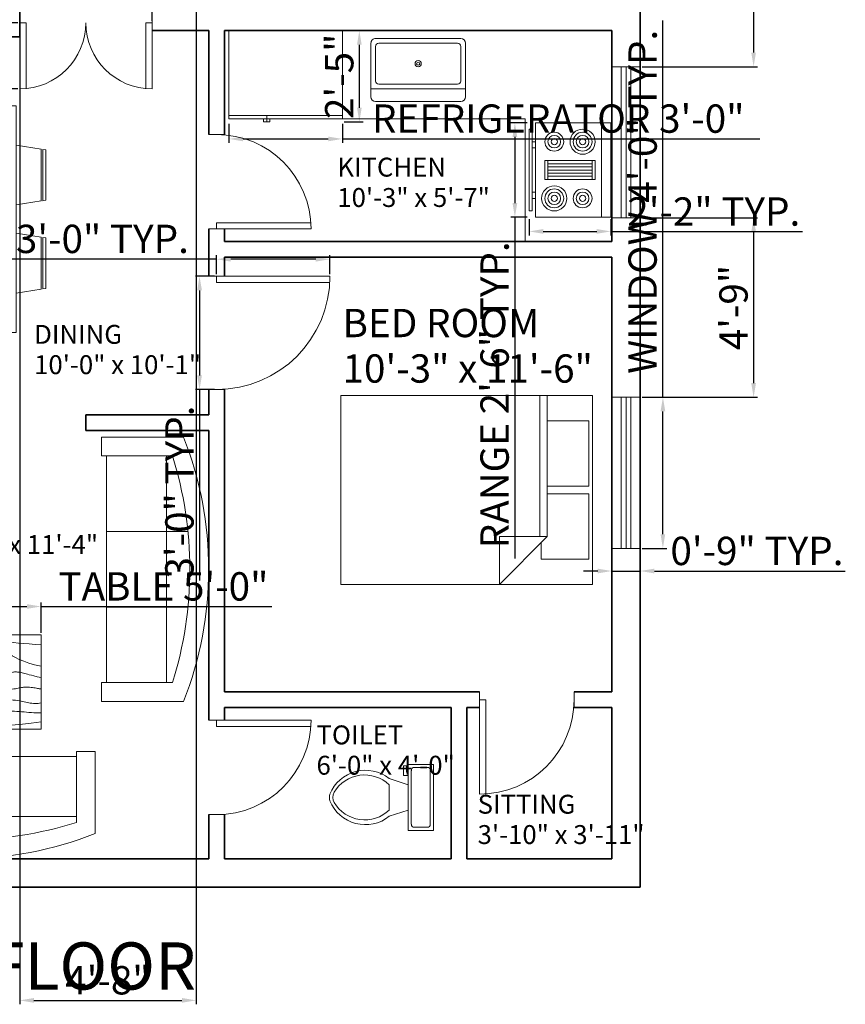
# Model space of a CAD drawing. Units: inches. Extents: x 3087 to 8148, y 1377 to 3709.
# Tile 4 of 6: x 3443 to 3705, y 1377 to 1689. Entities that reach past the tile are written whole.
import ezdxf

# ---------------------------------------------------------------- set-up
doc = ezdxf.new("R2010")
doc.units = ezdxf.units.IN
for name, color, linetype, lineweight, true_color in [('A-ANNO-DIMS', 244, 'Continuous', 18, 0x991b1e), ('A-ANNO-TEXT', 244, 'Continuous', 25, 0x991b1e), ('A-AREA-IDEN', 244, 'Continuous', 18, 0x991b1e), ('A-DOOR', 146, 'Continuous', 18, 0x105689), ('A-GLAZ', 146, 'Continuous', 18, 0x105689), ('A-WALL', 241, 'Continuous', 35, 0xf7abae)]:
    doc.layers.add(name, color=color, linetype=linetype, lineweight=lineweight, true_color=true_color)
for name, color, linetype, lineweight in [('A-EQPM', 8, 'Continuous', 18), ('A-FLOR-CASE', 9, 'Continuous', 18), ('A-FLOR-FIXT', 9, 'Continuous', 18), ('A-FURN', 8, 'Continuous', 18)]:
    doc.layers.add(name, color=color, linetype=linetype, lineweight=lineweight)
doc.styles.get("Standard").update_dxf_attribs({"font": 'arial.ttf'})
doc.dimstyles.new('ISO-25', dxfattribs={"dimtxt": 9, "dimasz": 4.5, "dimexe": 1.25, "dimexo": 0.625, "dimtad": 1, "dimdec": 0, "dimlunit": 3, "dimtxsty": 'Standard', "dimcen": 2.5, "dimadec": 0, "dimazin": 0, "dimtfac": 1, "dimtdec": 0, "dimtmove": 0, "dimatfit": 3, "dimfxl": 1, "dimarcsym": 0})

# ---------------------------------------------------------------- blocks, each defined once
blk = doc.blocks.new('Bed - Queen')
for p, q in [((0, -80.00003), (0, 0)), ((0, 0), (59.99999, 0)), ((59.99999, 0), (59.99999, -80.00003)), ((7.99999, -1.2), (28.79998, -1.2)), ((7.99999, -14.4), (7.99999, -1.2)), ((28.79998, -1.2), (28.79998, -14.4)), ((31.19999, -1.2), (51.99999, -1.2)), ((31.19999, -14.4), (31.19999, -1.2)), ((51.99999, -1.2), (51.99999, -16.4)), ((0, -14.4), (44.8, -14.4)), ((59.99999, -29.6), (44.8, -14.4)), ((44.8, -14.4), (44.8, -29.6)), ((44.8, -16.8), (0, -16.8)), ((51.99999, -16.4), (46.79936, -16.4)), ((44.8, -29.6), (59.99999, -29.6)), ((59.99999, -80.00003), (0, -80.00003))]:
    blk.add_line(p, q)
blk = doc.blocks.new('Sofa - Roundback 7 ft.')
for p, q in [((-12.00002, -32.4421), (-12.00003, -6.5971)), ((11.99997, -32.4421), (11.99998, -6.5971)), ((-36.000027, -34), (-36.000027, -11.4696)), ((35.99998, -34), (35.99998, -11.4696)), ((-35.999844, -13.3819), (35.9998, -13.3819)), ((-36.000027, -32.4421), (35.99998, -32.4421))]:
    blk.add_line(p, q)
for points in [[(-36.000027, -34), (-42.000027, -34), (-42.000027, -8)], [(41.99998, -8), (41.99998, -34), (35.99998, -34)]]:
    blk.add_lwpolyline(points)
for centre, radius, start, end in [((0, -114.25), 114.25, 68.43141, 111.5686), ((-0.00001, -127.1968), 121.1968, 72.72033, 107.2797)]:
    blk.add_arc(centre, radius, start, end)
blk = doc.blocks.new('Table - Rectangular Woodgrain 60 x 30 in.')
for p, q in [((0, 0), (0, -30)), ((60, 0), (0, 0)), ((60, -30), (60, 0)), ((0, -30), (60, -30))]:
    blk.add_line(p, q)
for points in [[(0, -2.4), (4.8155, -2.418), (9.0302, -2.4688), (12.709, -2.5477), (15.9167, -2.65), (18.7181, -2.7711), (21.1781, -2.9063), (23.3616, -3.0508), (25.3333, -3.2), (27.1477, -3.3495), (28.8172, -3.4958), (30.3437, -3.636), (31.7291, -3.7667), (32.9756, -3.8849), (34.0849, -3.9875), (35.059, -4.0714), (35.9, -4.1334), (36.6114, -4.1711), (37.2041, -4.1854), (37.6906, -4.1779), (38.0833, -4.15), (38.3948, -4.1034), (38.6375, -4.0396), (38.8239, -3.9602), (38.9666, -3.8667), (39.0764, -3.7608), (39.1573, -3.6448), (39.2116, -3.521), (39.2416, -3.3917), (39.2498, -3.2593), (39.2385, -3.1261), (39.21, -2.9944), (39.1666, -2.8667), (39.111, -2.7447), (39.0468, -2.6281), (38.978, -2.5163), (38.9083, -2.4083), (38.8418, -2.3035), (38.7823, -2.201), (38.7337, -2.1001), (38.7, -2), (38.6844, -1.9003), (38.6875, -1.8021), (38.7094, -1.707), (38.75, -1.6167), (38.8094, -1.5326), (38.8875, -1.4563), (38.9844, -1.3893), (39.1, -1.3333), (39.2351, -1.2896), (39.3937, -1.2583), (39.5804, -1.2396), (39.8, -1.2333), (40.057, -1.2396), (40.3562, -1.2583), (40.7023, -1.2896), (41.1, -1.3333), (41.5547, -1.3895), (42.0755, -1.4573), (42.6721, -1.5361), (43.3542, -1.625), (44.1316, -1.7233), (45.014, -1.8302), (46.0114, -1.9449), (47.1333, -2.0667), (48.3862, -2.1947), (49.7625, -2.3281), (51.2513, -2.4663), (52.8416, -2.6083), (54.5226, -2.7535), (56.2833, -2.9011), (58.1127, -3.0501), (60, -3.2)], [(0, -9.2), (6.5759, -9.0858), (11.9385, -9.0365), (16.2527, -9.0418), (19.6833, -9.0917), (22.3952, -9.1759), (24.5531, -9.2844), (26.322, -9.4069), (27.8666, -9.5333), (29.3241, -9.6553), (30.7203, -9.7719), (32.0532, -9.8837), (33.3208, -9.9917), (34.5213, -10.0965), (35.6526, -10.199), (36.7128, -10.2999), (37.7, -10.4), (38.6129, -10.4996), (39.4531, -10.5969), (40.223, -10.6895), (40.925, -10.775), (41.5613, -10.8512), (42.1344, -10.9156), (42.6465, -10.966), (43.1, -11), (43.4976, -11.0158), (43.8437, -11.0136), (44.143, -10.9942), (44.4, -10.9583), (44.6195, -10.9069), (44.8062, -10.8406), (44.9648, -10.7603), (45.1, -10.6667), (45.2155, -10.5598), (45.3114, -10.4365), (45.3871, -10.2929), (45.4416, -10.125), (45.4743, -9.929), (45.4844, -9.7011), (45.4709, -9.4371), (45.4333, -9.1333), (45.3716, -8.7883), (45.2896, -8.4104), (45.1919, -8.0107), (45.0833, -7.6), (44.9685, -7.1893), (44.8521, -6.7896), (44.7388, -6.4117), (44.6333, -6.0667), (44.54, -5.7628), (44.4614, -5.4979), (44.4001, -5.2675), (44.3583, -5.0667), (44.3384, -4.8909), (44.3427, -4.7354), (44.3736, -4.5956), (44.4333, -4.4667), (44.5236, -4.3453), (44.6427, -4.2333), (44.7884, -4.1339), (44.9583, -4.05), (45.1501, -3.9849), (45.3614, -3.9417), (45.59, -3.9234), (45.8333, -3.9333), (46.0915, -3.9749), (46.3734, -4.0531), (46.6906, -4.1736), (47.0542, -4.3417), (47.4756, -4.5629), (47.9661, -4.8427), (48.5372, -5.1866), (49.2, -5.6), (49.9676, -6.0844), (50.8594, -6.625), (51.8965, -7.2031), (53.1, -7.8), (54.491, -8.3969), (56.0906, -8.975), (57.9199, -9.5156), (60, -10)], [(0, -12.8), (5.1847, -12.9322), (9.6213, -13.0323), (13.3963, -13.1059), (16.5958, -13.1583), (19.3063, -13.1952), (21.614, -13.2219), (23.6054, -13.2439), (25.3666, -13.2667), (26.9728, -13.2947), (28.4531, -13.3281), (29.8256, -13.3663), (31.1083, -13.4083), (32.3191, -13.4535), (33.476, -13.501), (34.597, -13.5501), (35.7, -13.6), (36.7984, -13.6497), (37.8875, -13.6979), (38.9578, -13.743), (40, -13.7833), (41.0047, -13.8174), (41.9625, -13.8438), (42.864, -13.8607), (43.7, -13.8667), (44.4631, -13.8604), (45.1552, -13.8417), (45.7801, -13.8104), (46.3416, -13.7667), (46.8439, -13.7104), (47.2906, -13.6417), (47.6858, -13.5604), (48.0333, -13.4667), (48.3375, -13.3608), (48.6042, -13.2448), (48.8396, -13.121), (49.05, -12.9917), (49.2417, -12.8593), (49.4208, -12.7261), (49.5937, -12.5944), (49.7667, -12.4667), (49.9452, -12.3451), (50.1323, -12.2313), (50.3303, -12.1268), (50.5416, -12.0333), (50.7686, -11.9524), (51.0135, -11.8854), (51.2788, -11.8341), (51.5666, -11.8), (51.8785, -11.7843), (52.2116, -11.7865), (52.562, -11.8059), (52.926, -11.8417), (53.2998, -11.8931), (53.6795, -11.9594), (54.0614, -12.0397), (54.4416, -12.1333), (54.8223, -12.2401), (55.2293, -12.3625), (55.6942, -12.5037), (56.2489, -12.6667), (56.9251, -12.8547), (57.7545, -13.0708), (58.7689, -13.3182), (60, -13.6)], [(0, -18), (5.124, -17.7273), (9.6609, -17.5057), (13.6705, -17.3303), (17.2125, -17.1958), (20.3467, -17.0973), (23.1328, -17.0297), (25.6307, -16.9878), (27.9, -16.9667), (29.9928, -16.9617), (31.9302, -16.9703), (33.7254, -16.9907), (35.3917, -17.0208), (36.9423, -17.0588), (38.3906, -17.1026), (39.7499, -17.1503), (41.0333, -17.2), (42.2519, -17.2496), (43.4073, -17.2969), (44.4986, -17.3395), (45.525, -17.375), (46.4858, -17.4012), (47.3802, -17.4156), (48.2074, -17.416), (48.9667, -17.4), (49.6583, -17.3662), (50.2872, -17.3167), (50.8595, -17.2547), (51.3812, -17.1833), (51.8584, -17.1057), (52.2971, -17.025), (52.7034, -16.9443), (53.0833, -16.8667), (53.443, -16.7951), (53.789, -16.7313), (54.128, -16.6768), (54.4666, -16.6334), (54.8115, -16.6024), (55.1693, -16.5854), (55.5465, -16.5841), (55.95, -16.6), (56.3828, -16.6337), (56.8346, -16.6823), (57.2915, -16.7418), (57.7396, -16.8084), (58.165, -16.878), (58.5539, -16.9469), (58.8924, -17.0111), (59.1666, -17.0667), (59.3679, -17.1107), (59.5078, -17.1438), (59.6032, -17.1675), (59.6708, -17.1833), (59.7275, -17.193), (59.7901, -17.1979), (59.8753, -17.1998), (60, -17.2)], [(0, -22.4), (8.0098, -22.2501), (14.4094, -22.1011), (19.4168, -21.9535), (23.25, -21.8083), (26.1269, -21.6663), (28.2656, -21.5281), (29.884, -21.3947), (31.2, -21.2667), (32.3967, -21.1448), (33.5172, -21.0292), (34.5697, -20.9198), (35.5625, -20.8167), (36.5037, -20.7198), (37.4015, -20.6292), (38.2642, -20.5448), (39.1, -20.4667), (39.9164, -20.3951), (40.7187, -20.3313), (41.5117, -20.2768), (42.3, -20.2333), (43.0883, -20.2024), (43.8812, -20.1854), (44.6836, -20.1841), (45.5, -20.2), (46.3328, -20.234), (47.1747, -20.2844), (48.0163, -20.3488), (48.8479, -20.425), (49.66, -20.5106), (50.4429, -20.6031), (51.1872, -20.7004), (51.8833, -20.8), (52.5246, -20.8999), (53.1166, -20.9995), (53.6681, -21.0983), (54.1875, -21.1958), (54.6834, -21.2919), (55.1646, -21.3859), (55.6394, -21.4777), (56.1167, -21.5667), (56.6028, -21.6515), (57.0961, -21.7266), (57.5929, -21.7852), (58.0896, -21.8208), (58.5823, -21.8268), (59.0674, -21.7964), (59.5412, -21.723), (60, -21.6)], [(0, -25.2), (8.6355, -25.0504), (15.7026, -24.9031), (21.4049, -24.7606), (25.9458, -24.625), (29.529, -24.4988), (32.3578, -24.3844), (34.6359, -24.284), (36.5667, -24.2), (38.3213, -24.1341), (39.9417, -24.0854), (41.437, -24.0523), (42.8167, -24.0333), (44.0901, -24.0268), (45.2667, -24.0313), (46.3557, -24.0451), (47.3667, -24.0667), (48.309, -24.0947), (49.1928, -24.1287), (50.0284, -24.168), (50.826, -24.2125), (51.5959, -24.2617), (52.3483, -24.3151), (53.0935, -24.3725), (53.8417, -24.4334), (54.6009, -24.497), (55.3699, -24.561), (56.1454, -24.6226), (56.9239, -24.6792), (57.7021, -24.7279), (58.4764, -24.7662), (59.2435, -24.7911), (60, -24.8)], [(0, -28.8), (5.6867, -28.6681), (10.45, -28.5698), (14.407, -28.5012), (17.675, -28.4584), (20.3711, -28.4374), (22.6125, -28.4344), (24.5164, -28.4455), (26.2, -28.4667), (27.762, -28.4947), (29.2276, -28.5281), (30.6033, -28.5663), (31.8958, -28.6084), (33.1118, -28.6535), (34.2578, -28.7011), (35.3405, -28.7501), (36.3666, -28.8), (37.3443, -28.8497), (38.288, -28.8974), (39.2137, -28.9412), (40.1375, -28.9792), (41.0753, -29.0093), (42.0432, -29.0297), (43.0572, -29.0384), (44.1333, -29.0333), (45.2936, -29.0114), (46.5843, -28.9641), (48.0579, -28.8816), (49.7666, -28.7542), (51.7629, -28.5721), (54.0989, -28.3255), (56.8272, -28.0048), (60, -27.6)]]:
    blk.add_lwpolyline(points)
blk = doc.blocks.new('Toilet - top')
for p, q in [((9.5, -6), (9.5, -2)), ((-10, -8.5), (-8, -8.5)), ((-10, -9.5), (-10, -8.5)), ((-8, -8.5), (-8, -8)), ((-7, -8), (-7, -9.5)), ((-4, -8), (-6, -14)), ((4, -8), (6, -14)), ((-7, -9.5), (-10, -9.5)), ((4, -14), (-4, -14))]:
    blk.add_line(p, q)
blk.add_lwpolyline([(10.5, -8), (10.5, 0), (-10.5, 0), (-10.5, -8)], close=True)
for points in [[(-9.5, -2), (-9.5, -6)], [(8.5, -1), (-8.5, -1)], [(-8.5, -7), (8.5, -7)]]:
    blk.add_lwpolyline(points)
for centre, radius, start, end in [((-8.62, -1.88), 0.884, 81.8699, 188.1301), ((8.62, -1.88), 0.884, 351.8699, 98.1301), ((-8.62, -6.12), 0.884, 171.8699, 278.1301), ((8.62, -6.12), 0.884, 261.8699, 8.1301), ((3.52, -21.58), 12.17, 141.4691, 247.9714), ((4.2, -21.82), 11.33, 136.3677, 238.9468), ((-3.52, -21.58), 12.17, 292.0284, 38.5307), ((-4.2, -21.82), 11.33, 301.053, 43.6321), ((0, -27.88), 4, 245.7318, 294.2682), ((0, -29), 4, 254.8605, 285.1395)]:
    blk.add_arc(centre, radius, start, end)
blk = doc.blocks.new('Dining Set - 36 x 72 in.')
for p, q in [((-22.2343, 26.00059), (-23.4847, 17.99762)), ((-22.2304, 26), (-5.7608, 26)), ((-22, 27.5), (-22.1562, 26.50042)), ((-5.8416, 26.5), (-22.1534, 26.5)), ((-22, 27.5), (-6, 27.5)), ((-5.8437, 26.49966), (-6, 27.5)), ((-4.5152, 17.99762), (-5.7655, 25.99926)), ((5.7657, 26.00059), (4.5153, 17.99762)), ((5.7696, 26), (22.2392, 26)), ((6, 27.5), (5.8438, 26.50042)), ((22.1584, 26.5), (5.8466, 26.5)), ((6, 27.5), (22, 27.5)), ((22.1563, 26.49966), (22, 27.5)), ((23.4848, 17.99762), (22.2345, 25.99926)), ((36, 18), (-36, 18)), ((-36, 18), (-36, -18)), ((36, -18), (36, 18)), ((-44.0006, 8.23428), (-35.9976, 9.48474)), ((44.0006, 8.23428), (35.9976, 9.48474)), ((-45.5, 8), (-44.5004, 8.15617)), ((-45.5, 8), (-45.5, -8)), ((-44.5, -8.15843), (-44.5, 8.15338)), ((-44, 8.23041), (-44, -8.23915)), ((44, 8.23041), (44, -8.23915)), ((44.5, -8.15843), (44.5, 8.15338)), ((45.5, 8), (44.5005, 8.15617)), ((45.5, 8), (45.5, -8)), ((-44.4997, -8.15631), (-45.5, -8)), ((-35.9976, -9.48476), (-43.9993, -8.2345)), ((35.9976, -9.48476), (43.9993, -8.2345)), ((44.4997, -8.15631), (45.5, -8)), ((-36, -18), (36, -18)), ((-22.2343, -26.0006), (-23.4847, -17.99762)), ((-4.5152, -17.99762), (-5.7655, -25.99928)), ((5.7657, -26.0006), (4.5153, -17.99762)), ((23.4848, -17.99762), (22.2345, -25.99928)), ((-22.2304, -26), (-5.7608, -26)), ((-22, -27.5), (-22.1562, -26.50044)), ((-5.8416, -26.5), (-22.1534, -26.5)), ((-22, -27.5), (-6, -27.5)), ((-5.8437, -26.49967), (-6, -27.5)), ((5.7696, -26), (22.2392, -26)), ((6, -27.5), (5.8438, -26.50044)), ((22.1584, -26.5), (5.8466, -26.5)), ((6, -27.5), (22, -27.5)), ((22.1563, -26.49967), (22, -27.5))]:
    blk.add_line(p, q)
for points in [[(-36, 15), (-31.1772, 14.97754), (-26.8079, 14.91406), (-22.8538, 14.81543), (-19.276, 14.6875), (-16.0362, 14.53613), (-13.0957, 14.36718), (-10.4159, 14.18652), (-7.9583, 14), (-5.6904, 13.81315), (-3.6035, 13.63021), (-1.6954, 13.45508), (0.0365, 13.29166), (1.5945, 13.14388), (2.9811, 13.01562), (4.1988, 12.9108), (5.25, 12.83333), (6.1393, 12.78613), (6.8802, 12.76823), (7.4883, 12.77767), (7.9792, 12.8125), (8.3685, 12.87077), (8.6719, 12.95052), (8.9049, 13.0498), (9.0833, 13.16666), (9.2205, 13.29899), (9.3216, 13.44401), (9.3895, 13.59879), (9.4271, 13.76041), (9.4373, 13.92594), (9.4232, 14.09245), (9.3875, 14.257), (9.3333, 14.41666), (9.2638, 14.56917), (9.1836, 14.71484), (9.0975, 14.85465), (9.0104, 14.98958), (8.9272, 15.1206), (8.8529, 15.2487), (8.7922, 15.37483), (8.75, 15.5), (8.7305, 15.62467), (8.7344, 15.74739), (8.7617, 15.86621), (8.8125, 15.97916), (8.8867, 16.08431), (8.9844, 16.17968), (9.1055, 16.26334), (9.25, 16.33333), (9.4189, 16.38802), (9.6172, 16.42708), (9.8506, 16.45052), (10.125, 16.45833), (10.4463, 16.45052), (10.8203, 16.42708), (11.2529, 16.38802), (11.75, 16.33333), (12.3184, 16.26318), (12.9694, 16.17838), (13.7151, 16.07991), (14.5677, 15.96875), (15.5395, 15.84586), (16.6426, 15.71224), (17.8893, 15.56884), (19.2917, 15.41666), (20.859, 15.25667), (22.5879, 15.08984), (24.4721, 14.91715), (26.5052, 14.73958), (28.6809, 14.5581), (30.9929, 14.3737), (33.4347, 14.18733), (36, 14)], [(-36, 10), (-28.9766, 10.14274), (-23.1725, 10.20442), (-18.4241, 10.19775), (-14.5677, 10.13541), (-11.4399, 10.03011), (-8.877, 9.89453), (-6.7154, 9.74137), (-4.7917, 9.58333), (-2.9698, 9.43082), (-1.2246, 9.28515), (0.4415, 9.14534), (2.026, 9.01041), (3.5266, 8.87939), (4.9408, 8.7513), (6.266, 8.62516), (7.5, 8.5), (8.6411, 8.37549), (9.6914, 8.2539), (10.6538, 8.13818), (11.5312, 8.03125), (12.3267, 7.93603), (13.043, 7.85547), (13.6831, 7.79248), (14.25, 7.75), (14.7471, 7.7303), (15.1797, 7.73307), (15.5537, 7.75732), (15.875, 7.80208), (16.1494, 7.86637), (16.3828, 7.94922), (16.5811, 8.04964), (16.75, 8.16666), (16.8944, 8.29915), (17.0143, 8.44531), (17.1089, 8.60319), (17.1771, 8.77083), (17.218, 8.94629), (17.2305, 9.1276), (17.2137, 9.31282), (17.1667, 9.5), (17.0895, 9.6875), (16.987, 9.875), (16.8649, 10.0625), (16.7292, 10.25), (16.5856, 10.4375), (16.4401, 10.625), (16.2985, 10.8125), (16.1667, 11), (16.05, 11.18733), (15.9518, 11.3737), (15.8752, 11.5581), (15.8229, 11.73958), (15.798, 11.91715), (15.8034, 12.08984), (15.842, 12.25667), (15.9167, 12.41666), (16.0295, 12.56836), (16.1784, 12.70833), (16.3605, 12.83268), (16.5729, 12.9375), (16.8127, 13.01888), (17.0768, 13.07291), (17.3625, 13.0957), (17.6667, 13.08333), (17.9894, 13.03312), (18.3418, 12.94726), (18.7382, 12.82918), (19.1927, 12.68229), (19.7195, 12.51001), (20.3327, 12.31575), (21.0465, 12.10294), (21.875, 11.875), (22.8357, 11.63354), (23.959, 11.37304), (25.2786, 11.08618), (26.8282, 10.76562), (28.6414, 10.40405), (30.752, 9.99414), (33.1936, 9.52856), (36, 9)], [(-36, 5.5), (-30.7157, 5.3348), (-26.069, 5.20963), (-21.9946, 5.11767), (-18.4271, 5.05208), (-15.3009, 5.00602), (-12.5508, 4.97265), (-10.1112, 4.94515), (-7.9167, 4.91666), (-5.909, 4.88167), (-4.0586, 4.83984), (-2.3429, 4.79215), (-0.7396, 4.73958), (0.7739, 4.6831), (2.22, 4.6237), (3.6213, 4.56233), (5, 4.5), (6.373, 4.43782), (7.7344, 4.3776), (9.0723, 4.32129), (10.375, 4.27083), (11.6309, 4.22819), (12.8281, 4.19531), (13.9551, 4.17415), (15, 4.16666), (15.954, 4.17448), (16.819, 4.19791), (17.6001, 4.23698), (18.3021, 4.29166), (18.9299, 4.36198), (19.4883, 4.44791), (19.9823, 4.54948), (20.4167, 4.66666), (20.7969, 4.79899), (21.1302, 4.94401), (21.4245, 5.09879), (21.6875, 5.26041), (21.9271, 5.42594), (22.1511, 5.59245), (22.3672, 5.757), (22.5834, 5.91666), (22.8065, 6.06868), (23.0404, 6.21093), (23.2879, 6.34147), (23.5521, 6.45833), (23.8358, 6.55957), (24.142, 6.64323), (24.4735, 6.70735), (24.8334, 6.75), (25.2235, 6.76969), (25.642, 6.76692), (26.0858, 6.74267), (26.5521, 6.69791), (27.0379, 6.63362), (27.5404, 6.55078), (28.0565, 6.45036), (28.5834, 6.33333), (29.1242, 6.19987), (29.7071, 6.04687), (30.3661, 5.87044), (31.1354, 5.66666), (32.0493, 5.43164), (33.142, 5.16146), (34.4475, 4.85221), (36, 4.5)], [(-36, -1), (-30.7915, -0.6591), (-26.0195, -0.38216), (-21.6519, -0.16284), (-17.6563, 0.00521), (-14.0005, 0.12833), (-10.6523, 0.21289), (-7.5796, 0.26522), (-4.75, 0.29166), (-2.134, 0.29793), (0.2878, 0.28711), (2.5317, 0.26163), (4.6146, 0.22396), (6.5529, 0.17651), (8.3633, 0.12174), (10.0623, 0.06209), (11.6667, 0), (13.1899, -0.06201), (14.6341, -0.1211), (15.9982, -0.17432), (17.2813, -0.21875), (18.4823, -0.25147), (19.6003, -0.26953), (20.6343, -0.27002), (21.5834, -0.25), (22.4481, -0.20768), (23.2357, -0.14584), (23.9549, -0.06836), (24.6146, 0.02083), (25.2235, 0.11784), (25.7904, 0.21875), (26.3241, 0.31966), (26.8334, 0.41666), (27.3265, 0.50618), (27.8099, 0.58593), (28.2894, 0.65397), (28.7709, 0.70833), (29.2601, 0.74707), (29.763, 0.76823), (30.2855, 0.76985), (30.8334, 0.75), (31.4088, 0.70784), (31.9994, 0.64713), (32.589, 0.57275), (33.1615, 0.48958), (33.7008, 0.4025), (34.1908, 0.3164), (34.6153, 0.23616), (34.9584, 0.16666), (35.2099, 0.11165), (35.3848, 0.07031), (35.504, 0.04069), (35.5886, 0.02083), (35.6594, 0.00879), (35.7377, 0.0026), (35.8442, 0.00032), (36, 0)], [(-36, -6.5), (-27.1843, -6.31267), (-20.084, -6.1263), (-14.469, -5.9419), (-10.1094, -5.76042), (-6.7752, -5.58285), (-4.2363, -5.41016), (-2.2629, -5.24333), (-0.625, -5.08334), (0.8708, -4.93099), (2.2715, -4.78646), (3.5872, -4.64974), (4.8281, -4.52084), (6.0046, -4.39974), (7.127, -4.28646), (8.2053, -4.18099), (9.25, -4.08334), (10.2705, -3.99382), (11.2734, -3.91407), (12.2647, -3.84603), (13.25, -3.79167), (14.2354, -3.75293), (15.2266, -3.73177), (16.2295, -3.73015), (17.25, -3.75), (18.2912, -3.79248), (19.3451, -3.85547), (20.4009, -3.93604), (21.4479, -4.03125), (22.4754, -4.13819), (23.4727, -4.25391), (24.4289, -4.37549), (25.3334, -4.5), (26.1785, -4.62492), (26.9694, -4.74935), (27.7145, -4.87281), (28.4219, -4.99479), (29.1, -5.11483), (29.7572, -5.23242), (30.4016, -5.34709), (31.0417, -5.45834), (31.6837, -5.56437), (32.3262, -5.65821), (32.9658, -5.73153), (33.599, -5.77604), (34.2224, -5.78345), (34.8327, -5.74545), (35.4264, -5.65373), (36, -5.5)], [(-36, -10), (-26.4022, -9.81299), (-18.4675, -9.62891), (-11.9839, -9.45069), (-6.7396, -9.28125), (-2.5226, -9.12354), (0.8789, -8.98047), (3.6769, -8.85498), (6.0833, -8.75), (8.2767, -8.66765), (10.3021, -8.60677), (12.1712, -8.56543), (13.8958, -8.54167), (15.4876, -8.53353), (16.9583, -8.53907), (18.3197, -8.55632), (19.5834, -8.58334), (20.7616, -8.61841), (21.8685, -8.66081), (22.9188, -8.71004), (23.9271, -8.76563), (24.9081, -8.82707), (25.8763, -8.89388), (26.8465, -8.96558), (27.8334, -9.04167), (28.8474, -9.12118), (29.8828, -9.20117), (30.93, -9.27824), (31.9792, -9.34896), (33.0205, -9.40991), (34.0443, -9.45768), (35.0407, -9.48885), (36, -9.5)], [(-36, -14.5), (-30.0881, -14.33513), (-25.0332, -14.21224), (-20.7312, -14.12647), (-17.0781, -14.07292), (-13.97, -14.04671), (-11.3027, -14.04297), (-8.9724, -14.05681), (-6.875, -14.08334), (-4.9224, -14.11833), (-3.0905, -14.16016), (-1.3709, -14.20785), (0.2448, -14.26042), (1.7647, -14.3169), (3.1973, -14.3763), (4.5507, -14.43767), (5.8333, -14.5), (7.0554, -14.5621), (8.235, -14.62175), (9.3922, -14.67652), (10.5469, -14.72396), (11.7192, -14.76164), (12.929, -14.78711), (14.1965, -14.79794), (15.5417, -14.79167), (16.9933, -14.76424), (18.6152, -14.70508), (20.4804, -14.60197), (22.6615, -14.44271), (25.2312, -14.21509), (28.2624, -13.9069), (31.8277, -13.50594), (36, -13)]]:
    blk.add_lwpolyline(points)
blk = doc.blocks.new('Refrigerator-2 door - 36 in top')
for p, q in [((0, -26.999999), (36, -26.999999)), ((11, -27.999999), (11, -28.999999)), ((12, -26.999999), (12, -28.999999)), ((13, -28.999999), (13, -27.999999)), ((11, -28.999999), (13, -28.999999))]:
    blk.add_line(p, q)
blk.add_lwpolyline([(0, -27.999999), (0, 0), (36, 0), (36, -27.999999)], close=True)
blk = doc.blocks.new('Range-Oven - 30 in top')
for p, q in [((0, -3), (30, -3)), ((12, -6), (18, -6)), ((13, -20), (13, -6)), ((14, -6), (14, -20)), ((15, -20), (15, -6)), ((16, -6), (16, -20)), ((17, -20), (17, -6)), ((18, -20), (12, -20)), ((6, -24), (6, -25)), ((8, -25), (8, -24)), ((22, -25), (22, -24)), ((24, -24), (24, -25))]:
    blk.add_line(p, q)
for points in [[(0, -24), (0, 0), (30, 0), (30, -24)], [(12, -21), (12, -5), (18, -5), (18, -21)], [(2, -26), (2, -25), (28, -25), (28, -26)]]:
    blk.add_lwpolyline(points, close=True)
for centre, radius in [((6, -9), 4), ((6, -9), 3), ((24, -9), 3), ((6, -9), 2), ((6, -9), 1), ((24, -9), 2), ((24, -9), 1), ((6, -18), 3), ((24, -18), 4), ((24, -18), 3), ((6, -18), 2), ((6, -18), 1), ((24, -18), 2), ((24, -18), 1)]:
    blk.add_circle(centre, radius)
blk = doc.blocks.new('Sink-single - 30 in top')
blk.add_line((-15, -3.999996), (15, -3.999996))
for points in [[(-13.5, 0), (13.5, 0)], [(-15, -18.499996), (-15, -1.5)], [(15, -1.5), (15, -18.499996)], [(-12.5, -5.499996), (12.5, -5.499996)], [(-13.5, -17.499996), (-13.5, -6.499996)], [(13.5, -6.499996), (13.5, -17.499996)], [(12.5, -18.499996), (-12.5, -18.499996)], [(13.5, -19.999996), (-13.5, -19.999996)]]:
    blk.add_lwpolyline(points)
for radius in [1, 0.5]:
    blk.add_circle((0, -11.999996), radius)
for centre, radius, start, end in [((-13.5, -1.5), 1.5, 90, 180), ((13.5, -1.5), 1.5, 0, 90), ((-12.5, -6.499996), 1, 90, 180), ((12.5, -6.499996), 1, 0, 90), ((-13.5, -18.499996), 1.5, 180, 270), ((-12.5, -17.499996), 1, 180, 270), ((12.5, -17.499996), 1, 270, 0), ((13.5, -18.499996), 1.5, 270, 0)]:
    blk.add_arc(centre, radius, start, end)
blk = doc.blocks.new('DOOR-SINGLE-30IN')
for p, q in [((0, 30), (30, 30)), ((30, 30), (30, 28)), ((0, 28), (30, 28))]:
    blk.add_line(p, q)
blk.add_arc((30, 30), 30, 180, 270)
blk = doc.blocks.new('DOOR-SINGLE-36IN')
for p, q in [((0, 2), (36, 2)), ((36, 0), (36, 2)), ((0, 0), (36, 0))]:
    blk.add_line(p, q)
blk.add_arc((36, 0), 36, 90, 180)
blk = doc.blocks.new('DOOR-DOUBLE-42IN')
for p, q in [((0, 21), (0, 0)), ((2, 21), (2, 0)), ((40, 21), (40, 0)), ((42, 21), (42, 0)), ((0, 0), (2, 0)), ((42, 0), (40, 0))]:
    blk.add_line(p, q)
for centre, start, end in [((0, 0), 0, 90), ((42, 0), 90, 180)]:
    blk.add_arc(centre, 21, start, end)
blk = doc.blocks.new('WINDOW-48IN')
for p, q in [((0, 0), (0, 48)), ((0, 48), (9, 48)), ((3, 0), (3, 48)), ((4.5, 0), (4.5, 48)), ((6, 0), (6, 48)), ((9, 48), (9, 0)), ((9, 0), (0, 0))]:
    blk.add_line(p, q)
blk = doc.blocks.new('*D29')
at = {"layer": 'A-ANNO-DIMS', "color": 0, "lineweight": -2, "transparency": 16777216}
for p, q in [((3505.32, 1608.59), (3505.32, 1614.61)), ((3541.32, 1608.59), (3541.32, 1614.61)), ((3505.32, 1613.36), (3361.36, 1613.36)), ((3536.82, 1613.36), (3509.82, 1613.36))]:
    blk.add_line(p, q, dxfattribs=at)
at = {"layer": 'A-ANNO-DIMS', "color": 0, "transparency": 16777216}
for points in [[(3509.82, 1614.11), (3509.82, 1612.61), (3505.32, 1613.36)], [(3536.82, 1614.11), (3536.82, 1612.61), (3541.32, 1613.36)]]:
    blk.add_solid(points, dxfattribs=at)
at = {"layer": 'Defpoints', "color": 0, "transparency": 16777216}
for p in [(3505.32, 1613.36), (3505.32, 1607.96), (3541.32, 1607.96)]:
    blk.add_point(p, dxfattribs=at)
at = {"layer": 'A-ANNO-DIMS', "color": 0, "transparency": 16777216, "insert": (3431.09, 1618.65), "char_height": 9, "attachment_point": 5}
blk.add_mtext('ROOM DOOR 3\'-0" TYP.', dxfattribs=at)
blk = doc.blocks.new('*D30')
at = {"layer": 'A-ANNO-DIMS', "color": 0, "lineweight": -2, "transparency": 16777216}
for p, q in [((3504.69, 1607.96), (3498.67, 1607.96)), ((3499.92, 1603.46), (3499.92, 1576.46)), ((3504.69, 1571.96), (3498.67, 1571.96)), ((3499.92, 1571.96), (3499.92, 1511.36))]:
    blk.add_line(p, q, dxfattribs=at)
at = {"layer": 'A-ANNO-DIMS', "color": 0, "transparency": 16777216}
for points in [[(3499.17, 1603.46), (3500.67, 1603.46), (3499.92, 1607.96)], [(3499.17, 1576.46), (3500.67, 1576.46), (3499.92, 1571.96)]]:
    blk.add_solid(points, dxfattribs=at)
at = {"layer": 'Defpoints', "color": 0, "transparency": 16777216}
for p in [(3505.32, 1607.96), (3499.92, 1571.96), (3505.32, 1571.96)]:
    blk.add_point(p, dxfattribs=at)
at = {"layer": 'A-ANNO-DIMS', "color": 0, "transparency": 16777216, "insert": (3494.69, 1539.41), "char_height": 9, "attachment_point": 5, "rotation": 90}
blk.add_mtext('3\'-0" TYP.', dxfattribs=at)
blk = doc.blocks.new('*D39')
at = {"layer": 'A-ANNO-DIMS', "color": 0, "lineweight": -2, "transparency": 16777216}
for p, q in [((3647.02, 1569.52), (3647.02, 1689.16)), ((3640.44, 1569.52), (3648.27, 1569.52)), ((3647.02, 1526.02), (3647.02, 1565.02)), ((3640.44, 1521.52), (3648.27, 1521.52))]:
    blk.add_line(p, q, dxfattribs=at)
at = {"layer": 'A-ANNO-DIMS', "color": 0, "transparency": 16777216}
for points in [[(3646.27, 1565.02), (3647.77, 1565.02), (3647.02, 1569.52)], [(3646.27, 1526.02), (3647.77, 1526.02), (3647.02, 1521.52)]]:
    blk.add_solid(points, dxfattribs=at)
at = {"layer": 'Defpoints', "color": 0, "transparency": 16777216}
for p in [(3639.82, 1569.52), (3647.02, 1569.52), (3639.82, 1521.52)]:
    blk.add_point(p, dxfattribs=at)
at = {"layer": 'A-ANNO-DIMS', "color": 0, "transparency": 16777216, "insert": (3641.74, 1631.59), "char_height": 9, "attachment_point": 5, "rotation": 90}
blk.add_mtext('WINDOW 4\'-0" TYP.', dxfattribs=at)
blk = doc.blocks.new('*D40')
at = {"layer": 'A-ANNO-DIMS', "color": 0, "lineweight": -2, "transparency": 16777216}
for p, q in [((3630.82, 1520.9), (3630.82, 1513.07)), ((3639.82, 1520.9), (3639.82, 1513.07)), ((3626.32, 1514.32), (3621.82, 1514.32)), ((3630.82, 1514.32), (3639.82, 1514.32)), ((3644.32, 1514.32), (3704.93, 1514.32))]:
    blk.add_line(p, q, dxfattribs=at)
at = {"layer": 'A-ANNO-DIMS', "color": 0, "transparency": 16777216}
for points in [[(3626.32, 1515.07), (3626.32, 1513.57), (3630.82, 1514.32)], [(3644.32, 1515.07), (3644.32, 1513.57), (3639.82, 1514.32)]]:
    blk.add_solid(points, dxfattribs=at)
at = {"layer": 'Defpoints', "color": 0, "transparency": 16777216}
for p in [(3630.82, 1521.52), (3639.82, 1521.52), (3639.82, 1514.32)]:
    blk.add_point(p, dxfattribs=at)
at = {"layer": 'A-ANNO-DIMS', "color": 0, "transparency": 16777216, "insert": (3676.87, 1519.54), "char_height": 9, "attachment_point": 5}
blk.add_mtext('0\'-9" TYP.', dxfattribs=at)
blk = doc.blocks.new('*D45')
at = {"layer": 'A-ANNO-DIMS', "color": 0, "lineweight": -2, "transparency": 16777216}
for p, q in [((3603.9, 1656.69), (3598.78, 1656.69)), ((3600.03, 1652.19), (3600.03, 1631.19)), ((3603.9, 1626.69), (3598.78, 1626.69)), ((3600.03, 1626.69), (3600.03, 1518.35))]:
    blk.add_line(p, q, dxfattribs=at)
at = {"layer": 'A-ANNO-DIMS', "color": 0, "transparency": 16777216}
for points in [[(3599.28, 1652.19), (3600.78, 1652.19), (3600.03, 1656.69)], [(3599.28, 1631.19), (3600.78, 1631.19), (3600.03, 1626.69)]]:
    blk.add_solid(points, dxfattribs=at)
at = {"layer": 'Defpoints', "color": 0, "transparency": 16777216}
for p in [(3604.53, 1656.69), (3600.03, 1626.69), (3604.53, 1626.69)]:
    blk.add_point(p, dxfattribs=at)
at = {"layer": 'A-ANNO-DIMS', "color": 0, "transparency": 16777216, "insert": (3594.75, 1570.27), "char_height": 9, "attachment_point": 5, "rotation": 90}
blk.add_mtext('RANGE 2\'-6" TYP.', dxfattribs=at)
blk = doc.blocks.new('*D46')
at = {"layer": 'A-ANNO-DIMS', "color": 0, "lineweight": -2, "transparency": 16777216}
for p, q in [((3604.53, 1626.07), (3604.53, 1620.94)), ((3630.53, 1626.07), (3630.53, 1620.94)), ((3609.03, 1622.19), (3626.03, 1622.19)), ((3630.53, 1622.19), (3691.29, 1622.19))]:
    blk.add_line(p, q, dxfattribs=at)
at = {"layer": 'A-ANNO-DIMS', "color": 0, "transparency": 16777216}
for points in [[(3609.03, 1622.94), (3609.03, 1621.44), (3604.53, 1622.19)], [(3626.03, 1622.94), (3626.03, 1621.44), (3630.53, 1622.19)]]:
    blk.add_solid(points, dxfattribs=at)
at = {"layer": 'Defpoints', "color": 0, "transparency": 16777216}
for p in [(3604.53, 1626.69), (3630.53, 1626.69), (3630.53, 1622.19)]:
    blk.add_point(p, dxfattribs=at)
at = {"layer": 'A-ANNO-DIMS', "color": 0, "transparency": 16777216, "insert": (3663.16, 1627.34), "char_height": 9, "attachment_point": 5}
blk.add_mtext('2\'-2" TYP.', dxfattribs=at)
blk = doc.blocks.new('*D49')
at = {"layer": 'A-ANNO-DIMS', "color": 0, "lineweight": -2, "transparency": 16777216}
for p, q in [((3442.82, 1689.09), (3442.82, 1696.01)), ((3484.82, 1689.09), (3484.82, 1696.01)), ((3442.82, 1694.76), (3286.25, 1694.76)), ((3480.32, 1694.76), (3447.32, 1694.76))]:
    blk.add_line(p, q, dxfattribs=at)
at = {"layer": 'A-ANNO-DIMS', "color": 0, "transparency": 16777216}
for points in [[(3447.32, 1695.51), (3447.32, 1694.01), (3442.82, 1694.76)], [(3480.32, 1695.51), (3480.32, 1694.01), (3484.82, 1694.76)]]:
    blk.add_solid(points, dxfattribs=at)
at = {"layer": 'Defpoints', "color": 0, "transparency": 16777216}
for p in [(3442.82, 1694.76), (3442.82, 1688.46), (3484.82, 1688.46)]:
    blk.add_point(p, dxfattribs=at)
at = {"layer": 'A-ANNO-DIMS', "color": 0, "transparency": 16777216, "insert": (3362.28, 1700.05), "char_height": 9, "attachment_point": 5}
blk.add_mtext('DOUBLE DOOR 3\'-6" TYP.', dxfattribs=at)
blk = doc.blocks.new('*D50')
at = {"layer": 'A-ANNO-DIMS', "color": 0, "lineweight": -2, "transparency": 16777216}
for p, q in [((3442.19, 1688.46), (3435.27, 1688.46)), ((3436.52, 1683.96), (3436.52, 1671.96)), ((3442.19, 1667.46), (3435.27, 1667.46)), ((3436.52, 1667.46), (3436.52, 1607.7))]:
    blk.add_line(p, q, dxfattribs=at)
at = {"layer": 'A-ANNO-DIMS', "color": 0, "transparency": 16777216}
for points in [[(3435.77, 1683.96), (3437.27, 1683.96), (3436.52, 1688.46)], [(3435.77, 1671.96), (3437.27, 1671.96), (3436.52, 1667.46)]]:
    blk.add_solid(points, dxfattribs=at)
at = {"layer": 'Defpoints', "color": 0, "transparency": 16777216}
for p in [(3442.82, 1688.46), (3436.52, 1667.46), (3442.82, 1667.46)]:
    blk.add_point(p, dxfattribs=at)
at = {"layer": 'A-ANNO-DIMS', "color": 0, "transparency": 16777216, "insert": (3431.3, 1635.33), "char_height": 9, "attachment_point": 5, "rotation": 90}
blk.add_mtext('1\'-9" TYP.', dxfattribs=at)
blk = doc.blocks.new('*D51')
at = {"layer": 'A-ANNO-DIMS', "color": 0, "lineweight": -2, "transparency": 16777216}
for p, q in [((3389.59, 1494.68), (3389.59, 1504.31)), ((3449.59, 1494.68), (3449.59, 1504.31)), ((3394.09, 1503.06), (3445.09, 1503.06)), ((3449.59, 1503.06), (3522.82, 1503.06))]:
    blk.add_line(p, q, dxfattribs=at)
at = {"layer": 'A-ANNO-DIMS', "color": 0, "transparency": 16777216}
for points in [[(3394.09, 1503.81), (3394.09, 1502.31), (3389.59, 1503.06)], [(3445.09, 1503.81), (3445.09, 1502.31), (3449.59, 1503.06)]]:
    blk.add_solid(points, dxfattribs=at)
at = {"layer": 'Defpoints', "color": 0, "transparency": 16777216}
for p in [(3449.59, 1503.06), (3389.59, 1494.06), (3449.59, 1494.06)]:
    blk.add_point(p, dxfattribs=at)
at = {"layer": 'A-ANNO-DIMS', "color": 0, "transparency": 16777216, "insert": (3488.45, 1508.28), "char_height": 9, "attachment_point": 5}
blk.add_mtext('TABLE 5\'-0"', dxfattribs=at)
blk = doc.blocks.new('*D55')
at = {"layer": 'A-ANNO-DIMS', "color": 0, "lineweight": -2, "transparency": 16777216}
for p, q in [((3509.25, 1656.34), (3509.25, 1650.31)), ((3545.25, 1656.34), (3545.25, 1650.31)), ((3513.75, 1651.56), (3540.75, 1651.56)), ((3545.25, 1651.56), (3677.84, 1651.56))]:
    blk.add_line(p, q, dxfattribs=at)
at = {"layer": 'A-ANNO-DIMS', "color": 0, "transparency": 16777216}
for points in [[(3513.75, 1652.31), (3513.75, 1650.81), (3509.25, 1651.56)], [(3540.75, 1652.31), (3540.75, 1650.81), (3545.25, 1651.56)]]:
    blk.add_solid(points, dxfattribs=at)
at = {"layer": 'Defpoints', "color": 0, "transparency": 16777216}
for p in [(3509.25, 1656.96), (3545.25, 1656.96), (3545.25, 1651.56)]:
    blk.add_point(p, dxfattribs=at)
at = {"layer": 'A-ANNO-DIMS', "color": 0, "transparency": 16777216, "insert": (3613.79, 1656.85), "char_height": 9, "attachment_point": 5}
blk.add_mtext('REFRIGERATOR 3\'-0"', dxfattribs=at)
blk = doc.blocks.new('*D56')
at = {"layer": 'A-ANNO-DIMS', "color": 0, "lineweight": -2, "transparency": 16777216}
for p, q in [((3545.87, 1685.96), (3551.9, 1685.96)), ((3550.65, 1661.46), (3550.65, 1681.46)), ((3545.87, 1656.96), (3551.9, 1656.96))]:
    blk.add_line(p, q, dxfattribs=at)
at = {"layer": 'A-ANNO-DIMS', "color": 0, "transparency": 16777216}
for points in [[(3549.9, 1681.46), (3551.4, 1681.46), (3550.65, 1685.96)], [(3549.9, 1661.46), (3551.4, 1661.46), (3550.65, 1656.96)]]:
    blk.add_solid(points, dxfattribs=at)
at = {"layer": 'Defpoints', "color": 0, "transparency": 16777216}
for p in [(3545.25, 1685.96), (3550.65, 1685.96), (3545.25, 1656.96)]:
    blk.add_point(p, dxfattribs=at)
at = {"layer": 'A-ANNO-DIMS', "color": 0, "transparency": 16777216, "insert": (3545.43, 1671.46), "char_height": 9, "attachment_point": 5, "rotation": 90}
blk.add_mtext('2\'-5"', dxfattribs=at)
blk = doc.blocks.new('*D67')
at = {"layer": 'A-ANNO-DIMS', "color": 0, "lineweight": -2, "transparency": 16777216}
for p, q in [((3640.44, 1816.33), (3677.07, 1816.33)), ((3675.82, 1811.83), (3675.82, 1678.99)), ((3640.44, 1674.49), (3677.07, 1674.49))]:
    blk.add_line(p, q, dxfattribs=at)
at = {"layer": 'A-ANNO-DIMS', "color": 0, "transparency": 16777216}
for points in [[(3675.07, 1811.83), (3676.57, 1811.83), (3675.82, 1816.33)], [(3675.07, 1678.99), (3676.57, 1678.99), (3675.82, 1674.49)]]:
    blk.add_solid(points, dxfattribs=at)
at = {"layer": 'Defpoints', "color": 0, "transparency": 16777216}
for p in [(3639.82, 1816.33), (3639.82, 1674.49), (3675.82, 1674.49)]:
    blk.add_point(p, dxfattribs=at)
at = {"layer": 'A-ANNO-DIMS', "color": 0, "transparency": 16777216, "insert": (3670.6, 1745.41), "char_height": 9, "attachment_point": 5, "rotation": 90}
blk.add_mtext('11\'-10"', dxfattribs=at)
blk = doc.blocks.new('*D68')
at = {"layer": 'A-ANNO-DIMS', "color": 0, "lineweight": -2, "transparency": 16777216}
for p, q in [((3640.44, 1626.49), (3677.07, 1626.49)), ((3675.82, 1621.99), (3675.82, 1574.02)), ((3640.44, 1569.52), (3677.07, 1569.52))]:
    blk.add_line(p, q, dxfattribs=at)
at = {"layer": 'A-ANNO-DIMS', "color": 0, "transparency": 16777216}
for points in [[(3675.07, 1621.99), (3676.57, 1621.99), (3675.82, 1626.49)], [(3675.07, 1574.02), (3676.57, 1574.02), (3675.82, 1569.52)]]:
    blk.add_solid(points, dxfattribs=at)
at = {"layer": 'Defpoints', "color": 0, "transparency": 16777216}
for p in [(3639.82, 1626.49), (3639.82, 1569.52), (3675.82, 1569.52)]:
    blk.add_point(p, dxfattribs=at)
at = {"layer": 'A-ANNO-DIMS', "color": 0, "transparency": 16777216, "insert": (3670.6, 1598.01), "char_height": 9, "attachment_point": 5, "rotation": 90}
blk.add_mtext('4\'-9"', dxfattribs=at)
blk = doc.blocks.new('*D69')
at = {"layer": 'A-ANNO-DIMS', "color": 0, "lineweight": -2, "transparency": 16777216}
for p, q in [((3442.82, 1804.84), (3442.82, 1376.71)), ((3498.82, 1802.34), (3498.82, 1376.71)), ((3447.32, 1377.96), (3494.32, 1377.96))]:
    blk.add_line(p, q, dxfattribs=at)
at = {"layer": 'A-ANNO-DIMS', "color": 0, "transparency": 16777216}
for points in [[(3447.32, 1378.71), (3447.32, 1377.21), (3442.82, 1377.96)], [(3494.32, 1378.71), (3494.32, 1377.21), (3498.82, 1377.96)]]:
    blk.add_solid(points, dxfattribs=at)
at = {"layer": 'Defpoints', "color": 0, "transparency": 16777216}
for p in [(3442.82, 1805.46), (3498.82, 1802.96), (3498.82, 1377.96)]:
    blk.add_point(p, dxfattribs=at)
at = {"layer": 'A-ANNO-DIMS', "color": 0, "transparency": 16777216, "insert": (3470.82, 1383.18), "char_height": 9, "attachment_point": 5}
blk.add_mtext('4\'-8"', dxfattribs=at)

msp = doc.modelspace()

# ---------------------------------------------------------------- linework, layer by layer
at = {"layer": 'A-DOOR'}
for p, q in [((3484.82, 1685.96), (3484.82, 1690.96)), ((3507.82, 1652.96), (3502.82, 1652.96)), ((3507.82, 1622.96), (3502.82, 1622.96)), ((3507.82, 1607.96), (3502.82, 1607.96)), ((3507.82, 1571.96), (3502.82, 1571.96)), ((3588.82, 1470.96), (3588.82, 1475.96)), ((3618.82, 1470.96), (3618.82, 1475.96)), ((3507.82, 1466.96), (3502.82, 1466.96)), ((3507.82, 1436.96), (3502.82, 1436.96))]:
    msp.add_line(p, q, dxfattribs=at)
at = {"layer": 'A-FLOR-CASE'}
for p, q in [((3509.25, 1657.96), (3603.28, 1657.96)), ((3603.28, 1657.96), (3603.28, 1618.96))]:
    msp.add_line(p, q, dxfattribs=at)
at = {"layer": 'A-WALL'}
for p, q in [((3639.82, 2073.96), (3639.82, 1413.96)), ((3442.82, 1683.96), (3442.82, 1724.96)), ((3502.82, 1685.96), (3484.82, 1685.96)), ((3502.82, 1652.96), (3502.82, 1685.96)), ((3630.82, 1685.96), (3507.82, 1685.96)), ((3507.82, 1652.96), (3507.82, 1685.96)), ((3630.82, 1685.96), (3630.82, 1618.96)), ((3382.82, 1683.96), (3442.82, 1683.96)), ((3502.82, 1607.96), (3502.82, 1622.96)), ((3507.82, 1618.96), (3507.82, 1622.96)), ((3630.82, 1618.96), (3507.82, 1618.96)), ((3630.82, 1613.96), (3507.82, 1613.96)), ((3507.82, 1607.96), (3507.82, 1613.96)), ((3630.82, 1613.96), (3630.82, 1475.96)), ((3502.82, 1563.96), (3502.82, 1571.96)), ((3507.82, 1475.96), (3507.82, 1571.96)), ((3463.82, 1558.96), (3463.82, 1563.96)), ((3463.82, 1563.96), (3502.82, 1563.96)), ((3463.82, 1558.96), (3502.82, 1558.96)), ((3502.82, 1466.96), (3502.82, 1558.96)), ((3588.82, 1475.96), (3507.82, 1475.96)), ((3630.82, 1475.96), (3618.82, 1475.96)), ((3507.82, 1466.96), (3507.82, 1470.96)), ((3579.82, 1470.96), (3507.82, 1470.96)), ((3579.82, 1422.96), (3579.82, 1470.96)), ((3584.82, 1422.96), (3584.82, 1470.96)), ((3588.82, 1470.96), (3584.82, 1470.96)), ((3630.82, 1470.96), (3618.82, 1470.96)), ((3630.82, 1470.96), (3630.82, 1422.96)), ((3502.82, 1422.96), (3502.82, 1436.96)), ((3507.82, 1422.96), (3507.82, 1436.96)), ((3502.82, 1422.96), (3382.82, 1422.96)), ((3579.82, 1422.96), (3507.82, 1422.96)), ((3630.82, 1422.96), (3584.82, 1422.96)), ((3639.82, 1413.96), (3159.82, 1413.96))]:
    msp.add_line(p, q, dxfattribs=at)

# ---------------------------------------------------------------- block references
at = {"layer": 'A-DOOR'}
for name, p, rotation in [('DOOR-DOUBLE-42IN', (3484.82, 1688.46), 180), ('DOOR-SINGLE-30IN', (3535.32, 1652.96), 180), ('DOOR-SINGLE-36IN', (3541.32, 1607.96), 180), ('DOOR-SINGLE-30IN', (3618.82, 1443.46), 90.00000000000028)]:
    msp.add_blockref(name, p, dxfattribs=dict(at, rotation=rotation))
at = {"layer": 'A-DOOR', "extrusion": (0, 0, -1), "zscale": -1}
msp.add_blockref('DOOR-SINGLE-30IN', (-3535.32, 1436.96), dxfattribs=at)
at = {"layer": 'A-EQPM'}
msp.add_blockref('Refrigerator-2 door - 36 in top', (3509.25, 1685.96), dxfattribs=at)
at = {"layer": 'A-EQPM', "rotation": 270}
msp.add_blockref('Range-Oven - 30 in top', (3630.53, 1656.69), dxfattribs=at)
at = {"layer": 'A-FLOR-FIXT'}
for name, p, rotation in [('Sink-single - 30 in top', (3569.32, 1663.46), 180), ('Toilet - top', (3574.15, 1442.42), 270)]:
    msp.add_blockref(name, p, dxfattribs=dict(at, rotation=rotation))
at = {"layer": 'A-FURN'}
for name, p, rotation in [('Dining Set - 36 x 72 in.', (3423.66, 1626.1), 269.9999999999999), ('Bed - Queen', (3624.72, 1570.08), 270), ('Sofa - Roundback 7 ft.', (3502.82, 1514.88), 270), ('Sofa - Roundback 7 ft.', (3424.82, 1422.96), 180)]:
    msp.add_blockref(name, p, dxfattribs=dict(at, rotation=rotation))
msp.add_blockref('Table - Rectangular Woodgrain 60 x 30 in.', (3389.59, 1494.06), dxfattribs=at)
at = {"layer": 'A-GLAZ'}
for p in [(3630.82, 1626.49), (3630.82, 1521.52)]:
    msp.add_blockref('WINDOW-48IN', p, dxfattribs=at)

# ---------------------------------------------------------------- texts
at = {"layer": 'A-ANNO-TEXT'}
msp.add_text('FIRST AND SECOND FLOOR ', height=15, dxfattribs=at).set_placement((3241.85, 1381.38))
at = {"layer": 'A-AREA-IDEN'}
for s, height, p in [('KITCHEN', 6, (3543.64, 1639.6)), ('10\'-3" x 5\'-7"', 6, (3543.64, 1629.96)), ('BED ROOM ', 9, (3545.31, 1588.6)), ('DINING', 6, (3447.4, 1586.49)), ('10\'-0" x 10\'-1"', 6, (3447.4, 1576.86)), ('10\'-3" x 11\'-6"', 9, (3545.31, 1574.15)), ('10\'-0" x 11\'-4"', 6, (3414.7, 1519.74)), ('TOILET', 6, (3537.04, 1459.28)), ('6\'-0" x 4\'-0"', 6, (3537.04, 1449.64)), ('SITTING', 6, (3588.2, 1437.26)), ('3\'-10" x 3\'-11"', 6, (3588.2, 1427.62))]:
    msp.add_text(s, height=height, dxfattribs=at).set_placement(p)

# ---------------------------------------------------------------- dimensions: what is measured, and where the dimension line sits
at = {"layer": 'A-ANNO-DIMS'}
for base, p1, p2, picture, middle in [((3675.82, 1674.49), (3639.82, 1816.33), (3639.82, 1674.49), '*D67', (3670.6, 1745.41)), ((3550.65, 1685.96), (3545.25, 1656.96), (3545.25, 1685.96), '*D56', (3545.43, 1671.46)), ((3675.82, 1569.52), (3639.82, 1626.49), (3639.82, 1569.52), '*D68', (3670.6, 1598.01))]:
    dim = msp.add_linear_dim(base=base, p1=p1, p2=p2, angle=90, dimstyle='ISO-25', override={"dimdec": 1, "dimlfac": 1, "dimrnd": 0, "dimzin": 1, "dimdsep": 46, "dimlunit": 4, "dimfrac": 2}, dxfattribs=at)
    dim.commit()
    dim.dimension.update_dxf_attribs({"geometry": picture, "text_midpoint": middle})
dim = msp.add_linear_dim(base=(3498.82, 1377.96), p1=(3442.82, 1805.46), p2=(3498.82, 1802.96), dimstyle='ISO-25', override={"dimdec": 1, "dimlfac": 1, "dimrnd": 0, "dimzin": 1, "dimdsep": 46, "dimlunit": 4, "dimfrac": 2}, dxfattribs=at)
dim.commit()
dim.dimension.update_dxf_attribs({"geometry": '*D69', "text_midpoint": (3470.82, 1383.18)})
for base, p1, p2, angle, text, picture, middle in [((3442.82, 1694.76), (3484.82, 1688.46), (3442.82, 1688.46), 180, 'DOUBLE DOOR <> TYP.', '*D49', (3362.28, 1700.05)), ((3647.02, 1569.52), (3639.82, 1521.52), (3639.82, 1569.52), 90, 'WINDOW <> TYP.', '*D39', (3641.74, 1631.59)), ((3436.52, 1667.46), (3442.82, 1688.46), (3442.82, 1667.46), 270, '<> TYP.', '*D50', (3431.3, 1635.33)), ((3600.03, 1626.69), (3604.53, 1656.69), (3604.53, 1626.69), 270, 'RANGE <> TYP.', '*D45', (3594.75, 1570.27)), ((3505.32, 1613.36), (3541.32, 1607.96), (3505.32, 1607.96), 180, 'ROOM DOOR <> TYP.', '*D29', (3431.09, 1618.65)), ((3499.92, 1571.96), (3505.32, 1607.96), (3505.32, 1571.96), 270, '<> TYP.', '*D30', (3494.69, 1539.41))]:
    dim = msp.add_linear_dim(base=base, p1=p1, p2=p2, angle=angle, text=text, dimstyle='ISO-25', override={"dimdec": 1, "dimlfac": 1, "dimrnd": 0, "dimzin": 1, "dimdsep": 46, "dimlunit": 4, "dimfrac": 2}, dxfattribs=at)
    dim.commit()
    dim.dimension.update_dxf_attribs({"geometry": picture, "text_midpoint": middle})
for base, p1, p2, text, picture, middle in [((3545.25, 1651.56), (3509.25, 1656.96), (3545.25, 1656.96), 'REFRIGERATOR <>', '*D55', (3613.79, 1656.85)), ((3630.53, 1622.19), (3604.53, 1626.69), (3630.53, 1626.69), '<> TYP.', '*D46', (3663.16, 1627.34)), ((3639.82, 1514.32), (3630.82, 1521.52), (3639.82, 1521.52), '<> TYP.', '*D40', (3676.87, 1519.54)), ((3449.59, 1503.06), (3389.59, 1494.06), (3449.59, 1494.06), 'TABLE <>', '*D51', (3488.45, 1508.28))]:
    dim = msp.add_linear_dim(base=base, p1=p1, p2=p2, text=text, dimstyle='ISO-25', override={"dimdec": 1, "dimlfac": 1, "dimrnd": 0, "dimzin": 1, "dimdsep": 46, "dimlunit": 4, "dimfrac": 2}, dxfattribs=at)
    dim.commit()
    dim.dimension.update_dxf_attribs({"geometry": picture, "text_midpoint": middle})

doc.saveas('drawing.dxf')
